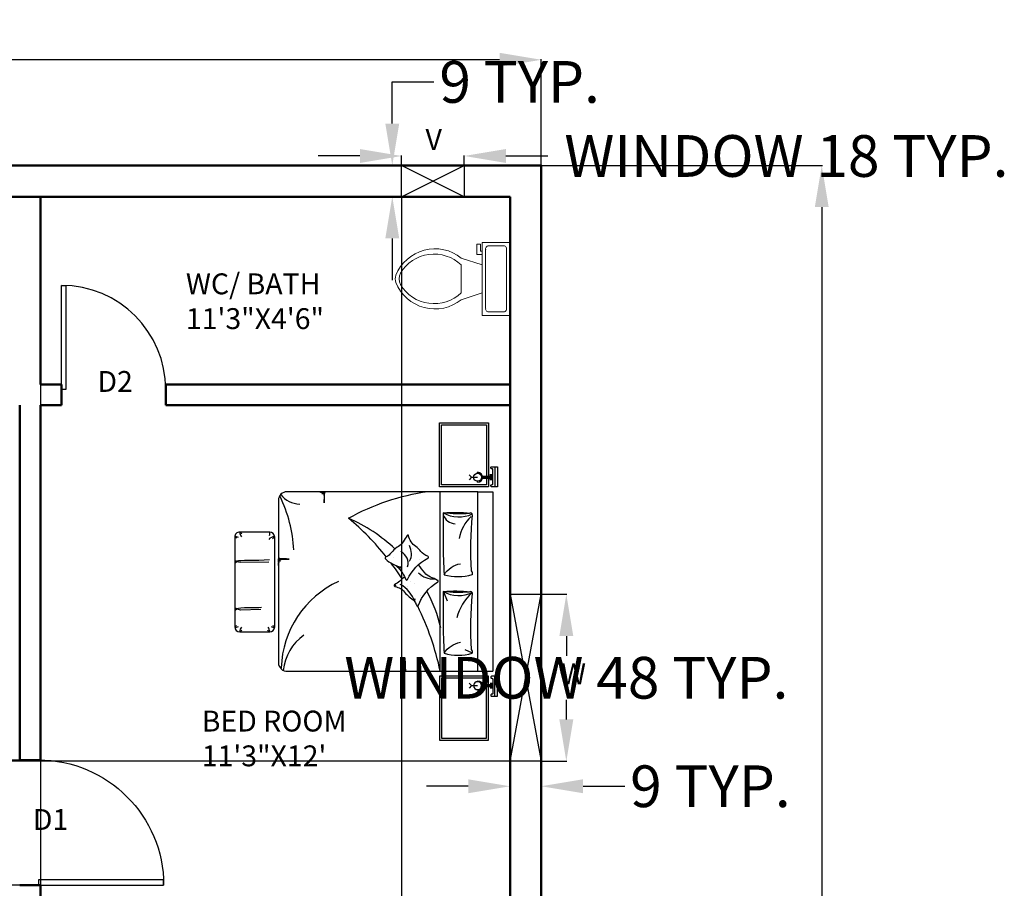
# Model space of a CAD drawing. Units: inches. Extents: x -77 to 516, y -119 to 536.
# Tile 11 of 11: x 224 to 507, y 287 to 536. Entities that reach past the tile are written whole.
import ezdxf

# ---------------------------------------------------------------- set-up
doc = ezdxf.new("R2010")
doc.units = ezdxf.units.IN
doc.header["$MEASUREMENT"] = 0
for name, color, linetype, lineweight in [('A-ANNO-DIMS', 2, 'Continuous', 18), ('A-AREA-IDEN', 170, 'Continuous', 25), ('A-FLOR-FIXT', 9, 'Continuous', 18), ('doors', 6, 'Continuous', 25), ('furniture', 119, 'Continuous', 18), ('text', 170, 'Continuous', 18), ('walls', 40, 'Continuous', 50), ('windows', 1, 'Continuous', 25)]:
    doc.layers.add(name, color=color, linetype=linetype, lineweight=lineweight)
for name, color, linetype in [('CEIL', 4, 'Continuous'), ('ELEC', 4, 'Continuous'), ('FUR', 42, 'Continuous'), ('wood', 26, 'Continuous')]:
    doc.layers.add(name, color=color, linetype=linetype)
doc.styles.get("Standard").update_dxf_attribs({"font": 'arial.ttf'})
doc.dimstyles.get("Standard").update_dxf_attribs({"dimtxt": 12, "dimasz": 12, "dimexe": 0.18, "dimexo": 0.0625, "dimgap": 0.09, "dimtad": 0, "dimtih": 1, "dimtoh": 1, "dimdec": 1, "dimzin": 0, "dimdsep": 46, "dimlunit": 4, "dimtxsty": 'Standard', "dimcen": 0.09, "dimadec": 0, "dimazin": 0, "dimtfac": 1, "dimtdec": 1, "dimtofl": 0, "dimtmove": 0, "dimatfit": 3, "dimfxl": 1, "dimtolj": 1, "dimtzin": 0, "dimarcsym": 0})

# ---------------------------------------------------------------- blocks, each defined once
blk = doc.blocks.new('*U2')
for p, q in [((0, 0), (0, -6)), ((40, 0), (40, -6))]:
    blk.add_line(p, q)
blk.add_lwpolyline([(0, 0), (0, 40), (1.75, 40), (1.75, 0)], close=True)
blk.add_arc((0, 0), 40, 0, 90)
blk = doc.blocks.new('*X12')
at = {"color": 0}
for p, q in [((3147.8, 8143.4), (3147.8, 8143.4)), ((3155.9, 8182.9), (3155.9, 8182.9)), ((3209.5, 8023.9), (3209.5, 8023.9)), ((3251.6, 7997), (3251.6, 7997)), ((3283, 8049.6), (3283, 8049.6)), ((3154.1, 7950.7), (3154.1, 7950.7))]:
    blk.add_line(p, q, dxfattribs=at)
blk = doc.blocks.new('*X11')
at = {"color": 0}
for p, q in [((3155.9, 8182.9), (3155.9, 8182.9)), ((3139.8, 7939.7), (3139.8, 7939.7))]:
    blk.add_line(p, q, dxfattribs=at)
blk = doc.blocks.new('*X10')
at = {"color": 0}
for p, q in [((3155.9, 8182.9), (3155.9, 8182.9)), ((3139.8, 7939.7), (3139.8, 7939.7))]:
    blk.add_line(p, q, dxfattribs=at)
blk = doc.blocks.new('*X9')
at = {"color": 0}
for p, q in [((3163, 7776.2), (3163, 7776.2)), ((3244.3, 7698.6), (3244.3, 7698.6)), ((3422.2, 7761.3), (3422.2, 7761.3)), ((3236.2, 7675.7), (3236.2, 7675.7)), ((3340.3, 7689.4), (3340.3, 7689.4))]:
    blk.add_line(p, q, dxfattribs=at)
blk = doc.blocks.new('BED1')
for p, q in [((0, -1000), (0, 800)), ((150, 800), (0, 800)), ((150, 800), (150, -1000)), ((2058.7, 800), (150, 800)), ((528, 800), (528, -1000)), ((211.8, 614.9), (277.5, 585.4)), ((2537.2, 404.9), (2237.2, 404.9)), ((2187.2, 354.9), (2187.2, -545.1)), ((2587.2, -545.1), (2587.2, 354.9)), ((2566.3, 178.5), (2565.2, 177.4)), ((2582, 188.1), (2565.4, 174.8)), ((2565.4, 174.8), (2585.7, 165.4)), ((2582, -287.1), (2565.4, -300.5)), ((2566.3, -296.8), (2565.2, -297.9)), ((2565.4, -300.5), (2585.7, -309.9)), ((2237.2, -595.1), (2537.2, -595.1)), ((150, -1000), (0, -1000)), ((150, -1000), (2063.5, -1000))]:
    blk.add_line(p, q)
for points in [[(934, 797.9), (930.9, 797.7), (928.3, 797.4), (926.3, 796.9), (924.9, 796.3), (923.8, 795.6), (923.1, 794.8), (922.7, 793.8), (922.5, 792.7), (922.4, 791.5), (922.5, 790.3), (922.6, 789.2), (922.6, 788.3), (922.6, 787.6), (922.4, 787.3), (922, 787.4), (921.4, 787.9), (920.6, 788.9), (919.5, 790.2), (918.4, 791.6), (917.1, 793.1), (915.9, 794.6), (914.6, 796), (913.3, 797.1), (912.2, 797.9), (911.1, 798.3), (910.1, 798.4), (909.2, 798), (908.3, 797.1), (907.5, 795.8), (906.8, 793.9), (906, 791.4), (905.4, 788.5), (904.8, 785.2), (904.2, 781.7), (903.7, 778.4), (903.2, 775.4), (902.8, 772.9), (902.5, 771.3), (902.3, 770.6), (902.1, 771.2), (902, 772.8), (901.8, 775.2), (901.7, 778.1), (901.5, 781.5), (901.2, 785), (900.8, 788.4), (900.2, 791.5), (899.5, 794.1), (898.6, 796.2), (897.6, 797.9), (896.5, 799.2), (895.3, 800), (894.1, 800.5), (893, 800.7), (891.9, 800.5), (890.9, 800.1), (890, 799), (889.1, 797.1), (888.3, 794), (887.6, 789.3), (886.9, 782.9), (886.2, 774.2), (885.5, 763.1), (884.8, 749.5), (884.2, 734.2), (883.6, 718.3), (883, 702.8), (882.5, 688.8), (882, 677.5), (881.7, 669.8), (881.5, 666.9), (881.3, 669.4), (881.3, 676.7), (881.3, 687.8), (881.2, 701.5), (881.1, 716.8), (880.8, 732.6), (880.2, 748), (879.4, 761.8), (878.3, 773.2), (876.9, 782.2), (875.1, 789.2), (872.9, 794.4), (870.3, 798), (869, 799)], [(2150, -913.5), (2150, 723.2)], [(2327.6, 182.3), (2530, 185.9), (2550.8, 181.9), (2561.7, 179), (2566, 176.7), (2566.9, 174.4), (2566.3, 171.9), (2562, 169.2), (2550.3, 166.5), (2527.7, 163.9), (2490.6, 161.8), (2345.5, 160.2), (2317.8, 158.5)], [(494.7, 3.1), (458.9, 95.3)], [(2149.7, -259.9), (2150, -268.4), (2150.1, -274.1), (2150.1, -278.1), (2150, -281.4), (2149.8, -284), (2149.5, -286.1), (2149.1, -287.8), (2148.7, -289), (2148.1, -289.9), (2147.4, -290.5), (2146.6, -290.8), (2145.6, -291), (2144.6, -291), (2143.6, -291), (2142.7, -290.9), (2141.9, -290.9), (2141.4, -290.9), (2141.1, -291), (2141.2, -291.4), (2141.7, -291.9), (2142.5, -292.6), (2143.5, -293.4), (2144.7, -294.4), (2146, -295.4), (2147.2, -296.5), (2148.4, -297.6), (2149.3, -298.6), (2150, -299.6), (2150.3, -300.5), (2150.4, -301.3), (2150, -302.1), (2149.3, -302.8), (2148.2, -303.5), (2146.6, -304.1), (2144.6, -304.7), (2142.1, -305.2), (2139.3, -305.7), (2136.5, -306.2), (2133.7, -306.6), (2131.2, -307), (2129.2, -307.3), (2127.8, -307.6), (2127.3, -307.8), (2127.7, -308), (2129, -308.1), (2131, -308.2), (2133.5, -308.3), (2136.3, -308.5), (2139.2, -308.7), (2142, -309), (2144.6, -309.5), (2146.8, -310.1), (2148.6, -310.9), (2150, -311.7), (2151, -312.7), (2151.7, -313.6), (2152.1, -314.6), (2152.3, -315.6), (2152.2, -316.5), (2151.8, -317.3), (2150.9, -318.1), (2149.3, -318.8), (2146.7, -319.4), (2142.8, -320), (2137.4, -320.6), (2130.2, -321.2), (2121, -321.8), (2109.7, -322.3), (2096.9, -322.9), (2083.6, -323.4), (2070.7, -323.9), (2059.1, -324.3), (2049.6, -324.7), (2043.2, -325), (2040.8, -325.2), (2042.9, -325.3), (2049, -325.3), (2058.2, -325.3), (2069.6, -325.4), (2082.3, -325.5), (2095.6, -325.8), (2108.4, -326.2), (2119.9, -326.8), (2129.4, -327.8), (2136.9, -329), (2142.7, -330.5), (2147, -332.3), (2150, -334.4), (2150.9, -335.6)], [(2246.5, -294.4), (2530, -289.4), (2550.8, -293.4), (2561.7, -296.3), (2566, -298.6), (2566.9, -300.8), (2566.3, -303.4), (2562, -306.1), (2550.3, -308.8), (2527.7, -311.3), (2490.6, -313.5), (2345.5, -315), (2238.6, -321.8)], [(1733.7, -998.3), (1731.1, -998.1), (1729, -997.8), (1727.4, -997.4), (1726.1, -997), (1725.2, -996.4), (1724.7, -995.7), (1724.3, -994.8), (1724.1, -993.9), (1724.1, -992.9), (1724.1, -991.9), (1724.2, -991), (1724.2, -990.2), (1724.2, -989.7), (1724.1, -989.4), (1723.8, -989.5), (1723.2, -990), (1722.5, -990.8), (1721.7, -991.8), (1720.7, -993), (1719.7, -994.3), (1718.6, -995.5), (1717.5, -996.6), (1716.5, -997.6), (1715.5, -998.3), (1714.6, -998.6), (1713.8, -998.6), (1713, -998.3), (1712.3, -997.6), (1711.7, -996.5), (1711, -994.9), (1710.4, -992.9), (1709.9, -990.4), (1709.4, -987.6), (1708.9, -984.8), (1708.5, -982), (1708.1, -979.5), (1707.8, -977.4), (1707.5, -976.1), (1707.3, -975.5), (1707.1, -976), (1707, -977.3), (1706.9, -979.3), (1706.8, -981.8), (1706.7, -984.6), (1706.4, -987.5), (1706.1, -990.3), (1705.6, -992.9), (1705, -995.1), (1704.2, -996.9), (1703.4, -998.3), (1702.4, -999.3), (1701.5, -1000), (1700.5, -1000.4), (1699.6, -1000.6), (1698.7, -1000.4), (1697.8, -1000.1), (1697, -999.2), (1696.3, -997.6), (1695.7, -995), (1695.1, -991.1), (1694.5, -985.7), (1693.9, -978.5), (1693.3, -969.3), (1692.8, -957.9), (1692.2, -945.2), (1691.7, -931.9), (1691.2, -919), (1690.8, -907.4), (1690.4, -897.9), (1690.1, -891.5), (1689.9, -889.1), (1689.8, -891.2), (1689.8, -897.3), (1689.8, -906.5), (1689.7, -917.9), (1689.6, -930.6), (1689.4, -943.8), (1688.9, -956.6), (1688.3, -968.1), (1687.3, -977.6), (1686.1, -985.2), (1684.6, -991), (1682.8, -995.3), (1680.7, -998.3), (1679.6, -999.2)]]:
    blk.add_lwpolyline(points)
for points in [[(205.5, 619.6, 0.267769), (215.1, 582.4, -0.037739), (204.3, 21.8, 0.684696), (236.7, 5.5, -0.060702), (497.2, 0.1, -0.046649), (225.9, 3.1, -1.318436)], [(489.2, 619.6, 0.144019), (207.6, 617.9, 0.248643)], [(497.2, 0.1, 0.021276), (489.2, 619.6, -0.206383), (326.6, 509.4, 0.237198)], [(211.8, 12.8, 0.143972), (361.6, 262.9, 1.292232)], [(886.4, -150, -0.069098), (985, -66.5, 0.658965), (982.1, -48.7, -0.049789), (927.4, -29, -0.103757), (896.6, -5.4, 0.055725), (800.9, 83.3, -0.11866), (782.7, 104.9, 0.016811), (761.6, 143.9, 0.70791), (748.3, 144, -0.16964), (551.9, -96.6, 0.664036), (554, -110.7, 0.023706), (627, -144.7, -0.134834), (683.2, -188, 0.012748), (746.3, -267.4)], [(205.5, -168.2, 0.267769), (215.1, -205.4, -0.037739), (204.3, -766, 0.684696), (236.7, -782.3, -0.060702), (497.2, -787.7, -0.046649), (225.9, -784.7, -1.318436)], [(489.2, -168.2, 0.144019), (207.6, -169.9, 0.248643)], [(497.2, -787.7, 0.021276), (489.2, -168.2, -0.206383), (326.6, -278.4, 0.237198)], [(969.1, -259.1, 0.263265), (936.3, -236.9, -0.026108), (909.2, -233.2, 0.027613), (945.1, -234.2, -0.089259), (872.7, -120, 0.662242), (857.6, -119.3, -0.162037), (651.8, -332.7, 0.676499), (654, -354.5, -0.160513), (722.9, -401.5, 0.07473), (773.5, -450.3, -0.187721), (845.5, -559.9, 0.70791), (858.8, -561.4, -0.010003), (898.6, -497.3, -0.113819), (947.3, -450.2, 0.099539), (1032.5, -372.4, -0.173425), (1070.9, -346.4, 0.589988), (1076.2, -326.1, 0.137312), (923.9, -245.9, 0.137312)], [(1446, -733.4, -0.095039), (652.8, -1001.7)]]:
    blk.add_lwpolyline(points, format="xyb")
for centre, radius, start, end in [((3208.8, 1363.3), 2739.4, 191.86791, 206.32469), ((1608.1, 842.5), 496.3, 305.19014, 354.02057), ((2062.7, 713.7), 86.5, 0, 93.53765), ((1138.6, 793.9), 983.2, 294.60777, 358.30329), ((2237.2, 354.9), 50, 90, 180), ((2321.1, 409.7), 84.5, 185.61958, 217.13957), ((2227.5, 373.5), 32.8, 17.83305, 72.80048), ((2546.9, 373.5), 32.8, 107.19952, 162.16695), ((2453.3, 409.7), 84.5, 322.86043, 354.38042), ((2537.2, 354.9), 50, 0, 90), ((2098.7, 754.7), 1625, 193.90497, 207.81692), ((2201.9, 323.3), 34.8, 50.8413, 114.9586), ((2212.2, 381.5), 36.5, 226.80948, 258.3841), ((2572.5, 323.3), 34.8, 65.0414, 129.1587), ((2562.2, 381.5), 36.5, 281.6159, 313.19052), ((751.8, 88.7), 34.9, 336.83517, 27.72181), ((684.2, 86), 100.3, 353.675, 10.88198), ((1074.1, 198.8), 306.1, 197.86019, 241.51221), ((341.4, -277.7), 318.5, 60.71255, 115.00895), ((983.7, -79.5), 20.8, 73.79673, 130.45661), ((978.5, -68.6), 14.3, 39.7097, 85.9506), ((602.5, -324), 198.6, 43.20348, 95.05559), ((3208.8, 1363.3), 2739.4, 212.93136, 216.95099), ((981.1, -281.8), 131.1, 164.0372, 243.45361), ((980, -379), 163.4, 152.61037, 209.36102), ((3208.8, 1363.3), 2739.4, 218.63292, 229.94485), ((2098.7, 754.7), 1625, 226.58872, 246.3156), ((3402.5, -342.9), 1408.5, 182.99169, 205.68187), ((-34.4, -471.2), 376.5, 312.01178, 350.96348), ((2178, -513.5), 33, 286.18268, 338.13858), ((2237.2, -545.1), 50, 180, 270), ((2188.1, -476.2), 73, 269.45125, 322.80265), ((2271.1, -580.9), 35.8, 148.90546, 197.55407), ((2546.9, -563.8), 32.8, 197.83305, 252.80048), ((2453.3, -600), 84.5, 5.61958, 37.13957), ((2537.2, -545.1), 50, 270, 0), ((2572.5, -513.6), 34.8, 230.8413, 294.9586), ((2562.2, -571.8), 36.5, 46.80948, 78.3841), ((375.7, -807.4), 128.2, 17.40732, 88.51286), ((341.4, -1065.5), 318.5, 60.71255, 115.00895), ((1929.1, -1126), 250.5, 37.85533, 88.44053), ((2063.5, -913.5), 86.5, 270, 0)]:
    blk.add_arc(centre, radius, start, end)
for name in ['*X11', '*X10', '*X12', '*X9']:
    blk.add_blockref(name, (-2425.3, -8101.4))
blk = doc.blocks.new('APLIQ')
at = {"layer": 'ELEC'}
for p, q in [((0, 0.2), (-0.0261, 0.2261)), ((0, 0.2), (0.0261, 0.2261)), ((0, 0.2), (0, 0.14)), ((-0.05, 0.14), (-0.04, 0.14)), ((0.04, 0.14), (0.05, 0.14)), ((-0.03, 0.01), (0.03, 0.01)), ((-0.03, 0), (0.03, 0)), ((-0.01, 0.09), (-0.01, 0.01)), ((0, 0.09), (0, 0)), ((0.01, 0.09), (0.01, 0.01))]:
    blk.add_line(p, q, dxfattribs=at)
blk.add_circle((0, 0.14), 0.04, dxfattribs=at)
blk.add_arc((0, 0.14), 0.05, 180, 0, dxfattribs=at)
blk = doc.blocks.new('A$C68AE1801')
at = {"layer": 'FUR'}
for points in [[(2.5416, 3.18), (2.5416, 2.54), (2.0516, 2.54), (2.0516, 3.18)], [(2.5216, 3.16), (2.5216, 2.56), (2.0716, 2.56), (2.0716, 3.16)], [(2.5416, 0), (2.5416, 0.64), (2.0516, 0.64), (2.0516, 0)], [(2.5216, 0.02), (2.5216, 0.62), (2.0716, 0.62), (2.0716, 0.02)]]:
    blk.add_lwpolyline(points, close=True, dxfattribs=at)
at = {"layer": 'wood'}
for p, q in [((2.6057, 2.74), (2.6057, 2.54)), ((2.6057, 0.44), (2.6057, 0.64))]:
    blk.add_line(p, q, dxfattribs=at)
for points in [[(2.5657, 2.728), (2.5657, 2.732, -0.414214), (2.5737, 2.74), (2.6321, 2.74), (2.6321, 2.54), (2.5737, 2.54, -0.414214), (2.5657, 2.548), (2.5657, 2.552, -0.414214), (2.5737, 2.56), (2.5777, 2.56, 0.414214), (2.5857, 2.568), (2.5857, 2.712, 0.414214), (2.5777, 2.72), (2.5737, 2.72, -0.414214)], [(2.5657, 0.452), (2.5657, 0.448, 0.414214), (2.5737, 0.44), (2.6321, 0.44), (2.6321, 0.64), (2.5737, 0.64, 0.414214), (2.5657, 0.632), (2.5657, 0.628, 0.414214), (2.5737, 0.62), (2.5777, 0.62, -0.414214), (2.5857, 0.612), (2.5857, 0.468, -0.414214), (2.5777, 0.46), (2.5737, 0.46, 0.414214)]]:
    blk.add_lwpolyline(points, format="xyb", close=True, dxfattribs=at)
at = {"layer": 'CEIL', "rotation": 90}
blk.add_blockref('APLIQ', (2.5736, 2.634), dxfattribs=at)
at = {"layer": 'CEIL', "xscale": -1, "rotation": 90}
blk.add_blockref('APLIQ', (2.5736, 0.546), dxfattribs=at)
at = {"layer": 'FUR', "xscale": 0.001, "yscale": 0.001, "zscale": 0.001, "rotation": 180}
blk.add_blockref('BED1', (2.5872, 1.49), dxfattribs=at)
blk = doc.blocks.new('*U16')
for p, q in [((9.5, -6), (9.5, -2)), ((-8, -8.5), (-8, -8)), ((-7, -8), (-7, -9.5)), ((-4, -8), (-6, -14)), ((4, -8), (6, -14)), ((-10, -8.5), (-8, -8.5)), ((-10, -9.5), (-10, -8.5)), ((-7, -9.5), (-10, -9.5)), ((4, -14), (-4, -14))]:
    blk.add_line(p, q)
blk.add_lwpolyline([(10.5, -8), (10.5, 0), (-10.5, 0), (-10.5, -8)], close=True)
for points in [[(-9.5, -2), (-9.5, -6)], [(8.5, -1), (-8.5, -1)], [(-8.5, -7), (8.5, -7)]]:
    blk.add_lwpolyline(points)
for centre, radius, start, end in [((-8.62, -1.88), 0.884, 81.8699, 188.1301), ((8.62, -1.88), 0.884, 351.8699, 98.1301), ((-8.62, -6.12), 0.884, 171.8699, 278.1301), ((8.62, -6.12), 0.884, 261.8699, 8.1301), ((3.52, -21.58), 12.17, 141.4691, 247.9714), ((4.2, -21.82), 11.33, 136.3677, 238.9468), ((-3.52, -21.58), 12.17, 292.0284, 38.5307), ((-4.2, -21.82), 11.33, 301.053, 43.6321), ((0, -27.88), 4, 245.7318, 294.2682), ((0, -29), 4, 254.8605, 285.1395)]:
    blk.add_arc(centre, radius, start, end)
blk = doc.blocks.new('WIN-48IN')
for p, q in [((0, 0), (9, 48)), ((0, 48), (9, 0))]:
    blk.add_line(p, q)
blk.add_lwpolyline([(0, 48), (9, 48), (9, 0), (0, 0)], close=True)
blk = doc.blocks.new('WIN-18IN')
for p, q in [((18, 0), (0, 9)), ((0, 0), (18, 9))]:
    blk.add_line(p, q)
blk.add_lwpolyline([(0, 9), (18, 9), (18, 0), (0, 0)], close=True)
blk = doc.blocks.new('*D22')
at = {"layer": 'A-ANNO-DIMS', "color": 0, "lineweight": -2, "transparency": 16777216}
for p, q in [((373.81, 371.24), (381.13, 371.24)), ((380.95, 359.24), (380.95, 353.54)), ((380.95, 335.24), (380.95, 340.94)), ((373.81, 323.24), (381.13, 323.24))]:
    blk.add_line(p, q, dxfattribs=at)
at = {"layer": 'A-ANNO-DIMS', "color": 0, "transparency": 16777216}
for points in [[(378.95, 359.24), (382.95, 359.24), (380.95, 371.24)], [(378.95, 335.24), (382.95, 335.24), (380.95, 323.24)]]:
    blk.add_solid(points, dxfattribs=at)
at = {"layer": 'Defpoints', "color": 0, "transparency": 16777216}
for p in [(373.75, 371.24), (380.95, 371.24), (373.75, 323.24)]:
    blk.add_point(p, dxfattribs=at)
at = {"layer": 'A-ANNO-DIMS', "color": 0, "transparency": 16777216, "insert": (380.95, 347.24), "char_height": 12, "attachment_point": 5}
blk.add_mtext('\\A1;WINDOW 48 TYP.', dxfattribs=at)
blk = doc.blocks.new('*D23')
at = {"layer": 'A-ANNO-DIMS', "color": 0, "lineweight": -2, "transparency": 16777216}
for p, q in [((364.75, 323.18), (364.75, 315.86)), ((373.75, 323.18), (373.75, 315.86)), ((352.75, 316.04), (340.75, 316.04)), ((385.75, 316.04), (397.75, 316.04))]:
    blk.add_line(p, q, dxfattribs=at)
at = {"layer": 'A-ANNO-DIMS', "color": 0, "transparency": 16777216}
for points in [[(352.75, 318.04), (352.75, 314.04), (364.75, 316.04)], [(385.75, 318.04), (385.75, 314.04), (373.75, 316.04)]]:
    blk.add_solid(points, dxfattribs=at)
at = {"layer": 'Defpoints', "color": 0, "transparency": 16777216}
for p in [(364.75, 323.24), (373.75, 323.24), (373.75, 316.04)]:
    blk.add_point(p, dxfattribs=at)
at = {"layer": 'A-ANNO-DIMS', "color": 0, "transparency": 16777216, "insert": (422.38, 316.04), "char_height": 12, "attachment_point": 5}
blk.add_mtext('\\A1;9 TYP.', dxfattribs=at)
blk = doc.blocks.new('*D24')
at = {"layer": 'A-ANNO-DIMS', "color": 0, "lineweight": -2, "transparency": 16777216}
for p, q in [((321.59, 497.29), (309.59, 497.29)), ((333.59, 494.65), (333.59, 497.47)), ((351.59, 494.65), (351.59, 497.47)), ((363.59, 497.29), (375.59, 497.29))]:
    blk.add_line(p, q, dxfattribs=at)
at = {"layer": 'A-ANNO-DIMS', "color": 0, "transparency": 16777216}
for points in [[(321.59, 499.29), (321.59, 495.29), (333.59, 497.29)], [(363.59, 499.29), (363.59, 495.29), (351.59, 497.29)]]:
    blk.add_solid(points, dxfattribs=at)
at = {"layer": 'Defpoints', "color": 0, "transparency": 16777216}
for p in [(351.59, 497.29), (333.59, 494.59), (351.59, 494.59)]:
    blk.add_point(p, dxfattribs=at)
at = {"layer": 'A-ANNO-DIMS', "color": 0, "transparency": 16777216, "insert": (444.24, 497.29), "char_height": 12, "attachment_point": 5}
blk.add_mtext('\\A1;WINDOW 18 TYP.', dxfattribs=at)
blk = doc.blocks.new('*D25')
at = {"layer": 'A-ANNO-DIMS', "color": 0, "lineweight": -2, "transparency": 16777216}
for p, q in [((330.89, 506.59), (330.89, 518.59)), ((330.89, 518.59), (342.89, 518.59)), ((333.53, 494.59), (330.71, 494.59)), ((333.53, 485.59), (330.71, 485.59)), ((330.89, 473.59), (330.89, 461.59))]:
    blk.add_line(p, q, dxfattribs=at)
at = {"layer": 'A-ANNO-DIMS', "color": 0, "transparency": 16777216}
for points in [[(328.89, 506.59), (332.89, 506.59), (330.89, 494.59)], [(328.89, 473.59), (332.89, 473.59), (330.89, 485.59)]]:
    blk.add_solid(points, dxfattribs=at)
at = {"layer": 'Defpoints', "color": 0, "transparency": 16777216}
for p in [(330.89, 494.59), (333.59, 494.59), (333.59, 485.59)]:
    blk.add_point(p, dxfattribs=at)
at = {"layer": 'A-ANNO-DIMS', "color": 0, "transparency": 16777216, "insert": (367.52, 518.59), "char_height": 12, "attachment_point": 5}
blk.add_mtext('\\A1;9 TYP.', dxfattribs=at)
blk = doc.blocks.new('*D36')
at = {"layer": 'A-ANNO-DIMS', "color": 0, "lineweight": -2, "transparency": 16777216}
for p, q in [((13.75, 494.65), (13.75, 525.13)), ((25.75, 524.95), (180.43, 524.95)), ((361.75, 524.95), (207.07, 524.95)), ((373.75, 494.65), (373.75, 525.13))]:
    blk.add_line(p, q, dxfattribs=at)
at = {"layer": 'A-ANNO-DIMS', "color": 0, "transparency": 16777216}
for points in [[(25.75, 526.95), (25.75, 522.95), (13.75, 524.95)], [(361.75, 526.95), (361.75, 522.95), (373.75, 524.95)]]:
    blk.add_solid(points, dxfattribs=at)
at = {"layer": 'Defpoints', "color": 0, "transparency": 16777216}
for p in [(373.75, 524.95), (13.75, 494.59), (373.75, 494.59)]:
    blk.add_point(p, dxfattribs=at)
at = {"layer": 'A-ANNO-DIMS', "color": 0, "transparency": 16777216, "insert": (193.75, 524.95), "char_height": 12, "attachment_point": 5}
blk.add_mtext('\\A1;360', dxfattribs=at)
blk = doc.blocks.new('*D37')
at = {"layer": 'A-ANNO-DIMS', "color": 0, "lineweight": -2, "transparency": 16777216}
for p, q in [((373.81, 494.59), (454.58, 494.59)), ((454.4, 482.59), (454.4, 212.81)), ((454.4, -69.41), (454.4, 200.37)), ((309, -81.41), (454.58, -81.41))]:
    blk.add_line(p, q, dxfattribs=at)
at = {"layer": 'A-ANNO-DIMS', "color": 0, "transparency": 16777216}
for points in [[(452.4, 482.59), (456.4, 482.59), (454.4, 494.59)], [(452.4, -69.41), (456.4, -69.41), (454.4, -81.41)]]:
    blk.add_solid(points, dxfattribs=at)
at = {"layer": 'Defpoints', "color": 0, "transparency": 16777216}
for p in [(373.75, 494.59), (454.4, 494.59), (308.93, -81.41)]:
    blk.add_point(p, dxfattribs=at)
at = {"layer": 'A-ANNO-DIMS', "color": 0, "transparency": 16777216, "insert": (454.4, 206.59), "char_height": 12, "attachment_point": 5}
blk.add_mtext('\\A1;576', dxfattribs=at)
blk = doc.blocks.new('*D41')
at = {"layer": 'A-ANNO-DIMS', "color": 0, "lineweight": -2, "transparency": 16777216}
for p, q in [((229.75, 485.53), (229.75, -111.24)), ((333.59, 485.53), (333.59, -111.24)), ((241.75, -111.06), (257.26, -111.06)), ((321.59, -111.06), (306.08, -111.06))]:
    blk.add_line(p, q, dxfattribs=at)
at = {"layer": 'A-ANNO-DIMS', "color": 0, "transparency": 16777216}
for points in [[(241.75, -109.06), (241.75, -113.06), (229.75, -111.06)], [(321.59, -109.06), (321.59, -113.06), (333.59, -111.06)]]:
    blk.add_solid(points, dxfattribs=at)
at = {"layer": 'Defpoints', "color": 0, "transparency": 16777216}
for p in [(229.75, 485.59), (333.59, 485.59), (333.59, -111.06)]:
    blk.add_point(p, dxfattribs=at)
at = {"layer": 'A-ANNO-DIMS', "color": 0, "transparency": 16777216, "insert": (281.67, -111.06), "char_height": 12, "attachment_point": 5}
blk.add_mtext('\\A1;103.84', dxfattribs=at)
blk = doc.blocks.new('*D46')
at = {"layer": 'A-ANNO-DIMS', "color": 0, "lineweight": -2, "transparency": 16777216}
for p, q in [((-15.9, 323.59), (-15.9, 335.59)), ((-15.9, 335.59), (-3.9, 335.59)), ((223.69, 323.59), (-16.08, 323.59)), ((-15.9, 299.59), (-15.9, 311.59)), ((223.69, 287.59), (-16.08, 287.59))]:
    blk.add_line(p, q, dxfattribs=at)
at = {"layer": 'A-ANNO-DIMS', "color": 0, "transparency": 16777216}
for points in [[(-17.9, 311.59), (-13.9, 311.59), (-15.9, 323.59)], [(-17.9, 299.59), (-13.9, 299.59), (-15.9, 287.59)]]:
    blk.add_solid(points, dxfattribs=at)
at = {"layer": 'Defpoints', "color": 0, "transparency": 16777216}
for p in [(-15.9, 323.59), (223.75, 323.59), (223.75, 287.59)]:
    blk.add_point(p, dxfattribs=at)
at = {"layer": 'A-ANNO-DIMS', "color": 0, "transparency": 16777216, "insert": (4.78, 335.59), "char_height": 12, "attachment_point": 5}
blk.add_mtext('\\A1;36', dxfattribs=at)
blk = doc.blocks.new('*D48')
at = {"layer": 'A-ANNO-DIMS', "color": 0, "lineweight": -2, "transparency": 16777216}
for p, q in [((364.69, 323.24), (-16.08, 323.24)), ((-15.9, 311.24), (-15.9, 308.63)), ((-15.9, 293.59), (-15.9, 296.2)), ((364.69, 281.59), (-16.08, 281.59))]:
    blk.add_line(p, q, dxfattribs=at)
at = {"layer": 'A-ANNO-DIMS', "color": 0, "transparency": 16777216}
for points in [[(-17.9, 311.24), (-13.9, 311.24), (-15.9, 323.24)], [(-17.9, 293.59), (-13.9, 293.59), (-15.9, 281.59)]]:
    blk.add_solid(points, dxfattribs=at)
at = {"layer": 'Defpoints', "color": 0, "transparency": 16777216}
for p in [(-15.9, 323.24), (364.75, 323.24), (364.75, 281.59)]:
    blk.add_point(p, dxfattribs=at)
at = {"layer": 'A-ANNO-DIMS', "color": 0, "transparency": 16777216, "insert": (-15.9, 302.42), "char_height": 12, "attachment_point": 5}
blk.add_mtext('\\A1;41.65', dxfattribs=at)

msp = doc.modelspace()

# ---------------------------------------------------------------- linework, layer by layer
at = {"layer": 'walls'}
for p, q in [((364.7501, 485.5884), (22.7501, 485.5884)), ((229.7501, 485.5884), (229.7501, 431.5884)), ((364.7501, 131.5884), (364.7501, 485.5884)), ((235.7501, 431.5884), (229.7501, 431.5884)), ((235.7501, 431.5884), (235.7501, 425.5884)), ((364.7501, 431.5884), (265.7501, 431.5884)), ((265.7501, 431.5884), (265.7501, 425.5884)), ((223.7501, 425.5884), (223.7501, 323.5884)), ((235.7501, 425.5884), (229.7501, 425.5884)), ((229.7501, 425.5884), (229.7501, 323.5884)), ((364.7501, 425.5884), (265.7501, 425.5884)), ((229.7501, 323.5884), (223.7501, 323.5884)), ((229.7501, 287.5884), (223.7501, 287.5884)), ((229.7501, 287.5884), (229.7501, 281.5884))]:
    msp.add_line(p, q, dxfattribs=at)
msp.add_lwpolyline([(373.7501, 131.5884), (373.7501, 494.5884), (13.7501, 494.5884), (13.7501, 14.5884), (239.7501, 14.5884)], dxfattribs=at)

# ---------------------------------------------------------------- block references
at = {"layer": 'A-FLOR-FIXT', "rotation": 270}
msp.add_blockref('*U16', (364.7501, 461.949), dxfattribs=at)
at = {"layer": 'doors', "xscale": 0.7499999999999986, "yscale": 0.7499999999999986, "zscale": 0.7499999999999986}
msp.add_blockref('*U2', (235.7501, 430.0884), dxfattribs=at)
at = {"layer": 'doors', "xscale": -0.9, "yscale": 0.9, "zscale": 0.9, "rotation": 270}
msp.add_blockref('*U2', (229.1501, 287.5884), dxfattribs=at)
at = {"layer": 'furniture', "xscale": 28.69583594835296, "yscale": 28.69583594835296, "zscale": 28.69583594835296}
msp.add_blockref('A$C68AE1801', (285.599, 329.2997), dxfattribs=at)
at = {"layer": 'windows'}
for name, p in [('WIN-18IN', (333.5884, 485.588)), ('WIN-48IN', (364.75, 323.2431))]:
    msp.add_blockref(name, p, dxfattribs=at)

# ---------------------------------------------------------------- texts
at = {"layer": 'A-AREA-IDEN', "char_height": 6, "attachment_point": 1}
for s, insert in [('WC/ BATH\\P11\'3"X4\'6"', (271.5513, 463.5191)), ('BED ROOM\\P11\'3"X12\'', (276.1097, 337.7807))]:
    msp.add_mtext_dynamic_manual_height_columns(s, width=105.041962, gutter_width=1, heights=[0], dxfattribs=dict(at, insert=insert))
at = {"layer": 'text', "char_height": 6, "attachment_point": 1}
for s, insert in [('V ', (340.4537, 505.0267)), ('D2', (246.1038, 435.4469)), ('W', (379.4204, 351.3535)), ('D1', (227.552, 309.476))]:
    msp.add_mtext_dynamic_manual_height_columns(s, width=105.041962, gutter_width=1, heights=[0], dxfattribs=dict(at, insert=insert))

# ---------------------------------------------------------------- dimensions: what is measured, and where the dimension line sits
at = {"layer": 'A-ANNO-DIMS'}
for base, p1, p2, text, picture, middle in [((330.8885, 494.5884), (333.5885, 485.5884), (333.5885, 494.5884), '<> TYP.', '*D25', (367.5228, 518.5884)), ((380.9501, 371.2426), (373.7501, 323.2426), (373.7501, 371.2426), 'WINDOW <> TYP.', '*D22', (380.9501, 347.2426))]:
    dim = msp.add_linear_dim(base=base, p1=p1, p2=p2, angle=90, text=text, dimstyle='Standard', override={"dimdec": 0, "dimlfac": 1, "dimrnd": 0, "dimzin": 0, "dimdsep": 46, "dimlunit": 2}, dxfattribs=at)
    dim.commit()
    dim.dimension.update_dxf_attribs({"geometry": picture, "text_midpoint": middle})
for base, p1, p2, override, picture, middle in [((373.7501, 524.9457), (13.7501, 494.5884), (373.7501, 494.5884), {"dimdec": 0, "dimlfac": 1, "dimrnd": 0, "dimzin": 0, "dimdsep": 46, "dimlunit": 2}, '*D36', (193.7501, 524.9457)), ((333.5885, -111.0616), (229.7501, 485.5884), (333.5885, 485.5884), {"dimdec": 2, "dimlfac": 1, "dimrnd": 0, "dimzin": 0, "dimdsep": 46, "dimlunit": 2}, '*D41', (281.6693, -111.0616))]:
    dim = msp.add_linear_dim(base=base, p1=p1, p2=p2, dimstyle='Standard', override=override, dxfattribs=at)
    dim.commit()
    dim.dimension.update_dxf_attribs({"geometry": picture, "text_midpoint": middle})
for base, p1, p2, text, picture, middle in [((351.5885, 497.2884), (333.5885, 494.5884), (351.5885, 494.5884), 'WINDOW <> TYP.', '*D24', (444.2365, 497.2884)), ((373.7501, 316.0426), (364.7501, 323.2426), (373.7501, 323.2426), '<> TYP.', '*D23', (422.3844, 316.0426))]:
    dim = msp.add_linear_dim(base=base, p1=p1, p2=p2, text=text, dimstyle='Standard', override={"dimdec": 0, "dimlfac": 1, "dimrnd": 0, "dimzin": 0, "dimdsep": 46, "dimlunit": 2}, dxfattribs=at)
    dim.commit()
    dim.dimension.update_dxf_attribs({"geometry": picture, "text_midpoint": middle})
for base, p1, p2, override, picture, middle in [((454.4001, 494.5884), (308.9336, -81.4116), (373.7501, 494.5884), {"dimdec": 0, "dimlfac": 1, "dimrnd": 0, "dimzin": 0, "dimdsep": 46, "dimlunit": 2}, '*D37', (454.4001, 206.5884)), ((-15.8999, 323.5884), (223.7501, 287.5884), (223.7501, 323.5884), {"dimdec": 0, "dimlfac": 1, "dimrnd": 0, "dimzin": 0, "dimdsep": 46, "dimlunit": 2}, '*D46', (4.7767, 335.5884)), ((-15.8999, 323.2426), (364.7501, 281.5884), (364.7501, 323.2426), {"dimdec": 2, "dimlfac": 1, "dimrnd": 0, "dimzin": 0, "dimdsep": 46, "dimlunit": 2}, '*D48', (-15.8999, 302.4155))]:
    dim = msp.add_linear_dim(base=base, p1=p1, p2=p2, angle=90, dimstyle='Standard', override=override, dxfattribs=at)
    dim.commit()
    dim.dimension.update_dxf_attribs({"geometry": picture, "text_midpoint": middle})

doc.saveas('drawing.dxf')
